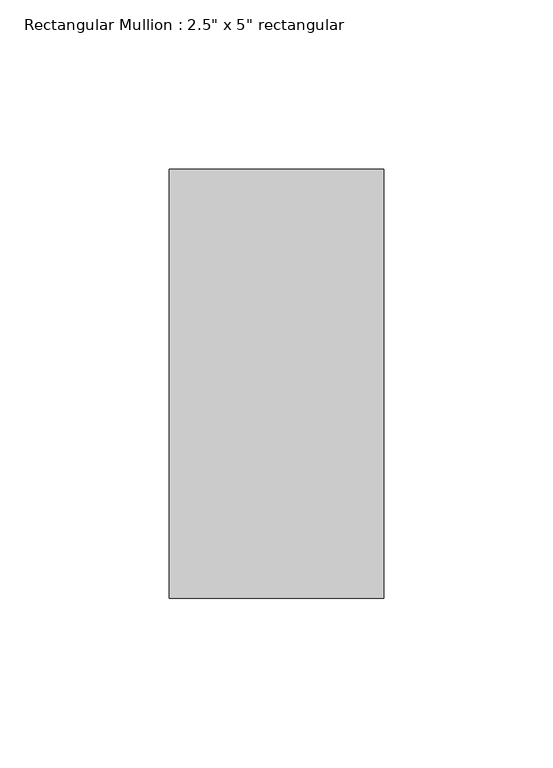
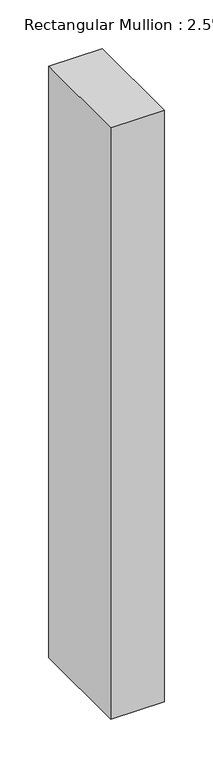
"""IFC4 building model written with IfcOpenShell, lengths in millimetres: member geometry."""

from ifc_helpers import new_model, si_unit, frame, origin, place, context, project, spatial, polyline, outline, extrude, source, transform, mapped, element, save


def member_f89ab80f(model_context):
    return source(origin(), model_context, "Body", "SweptSolid", [
        extrude(outline(polyline([(0.0, 63.5), (0.0, -63.5), (-63.5, -63.5), (-63.5, 63.5), (0.0, 63.5)])), frame((0.0, 0.0, -740.8042001), z_axis=(0.0, 0.0, 1.0), x_axis=(1.0, 0.0, 0.0)), (0.0, 0.0, 1.0), 740.8042001),
    ])


if __name__ == "__main__":
    model = new_model("IFC4")
    model_context = context("Model", 3, world=origin())
    ifc_project = project(units=[si_unit("LENGTHUNIT", "METRE", prefix="MILLI")], contexts=[model_context])
    site = spatial("IfcSite", under=ifc_project)
    building = spatial("IfcBuilding", under=site)
    placement = place(None, origin())
    member_shape = member_f89ab80f(model_context)
    element("IfcMember", 1, ObjectType="Rectangular Mullion : 2.5\" x 5\" rectangular", at=placement, inside=building, context=model_context, shape_type="MappedRepresentation", body=[
        mapped(member_shape, transform((0.0, 0.0, 0.0), x_axis=(1.0, 0.0, 0.0), y_axis=(0.0, 1.0, 0.0), z_axis=(0.0, 0.0, 1.0))),
    ])
    save(model, "model.ifc")

# Revit data of these elements
# Type "Rectangular Mullion : 2.5\" x 5\" rectangular"
#   built-in parameter 1007304 = 0.416667 (stored number, unit not read)
#   built-in parameter 1007301 = 0.104167 (stored number, unit not read)
#   built-in parameter 1007300 = 0.104167 (stored number, unit not read)
# Element 1 (IfcMember, "Rectangular Mullion : 2.5\" x 5\" rectangular")
#   Materials on its faces: "Aluminum"
# Materials
#   "Aluminum": class "Metal", colour RGB 247 247 247, transparency 0, Description = "Aluminum 6061", Cost = 0
